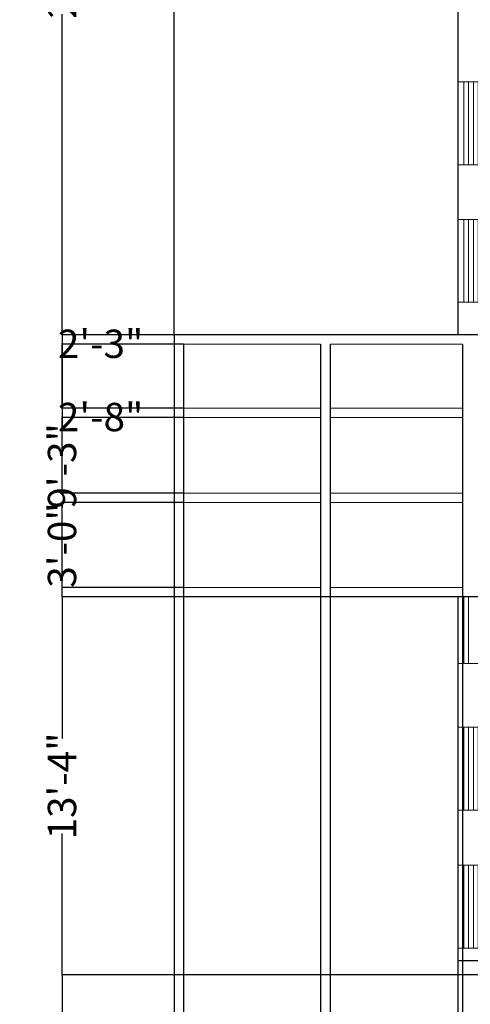
# Model space of a CAD drawing. Units: inches. Extents: x 1146 to 2917, y 889 to 2437.
# Tile 11 of 13: x 2395 to 2585, y 1586 to 2003. Entities that reach past the tile are written whole.
import ezdxf

# ---------------------------------------------------------------- set-up
doc = ezdxf.new("R2010")
doc.units = ezdxf.units.IN
doc.header["$MEASUREMENT"] = 0
for name, color, linetype, lineweight in [('A-ANNO-DIMS', 2, 'Continuous', 18), ('A-ELEV', 7, 'Continuous', 30), ('A-ELEV-GLAZ', 5, 'Continuous', 18), ('A-ELEV-ORNM', 8, 'Continuous', 18)]:
    doc.layers.add(name, color=color, linetype=linetype, lineweight=lineweight)
doc.styles.get("Standard").update_dxf_attribs({"font": 'arial.ttf'})
doc.dimstyles.get("Standard").update_dxf_attribs({"dimtxt": 12, "dimasz": 0.18, "dimexe": 0.18, "dimexo": 0.0625, "dimgap": 0.09, "dimtad": 0, "dimtoh": 1, "dimdec": 1, "dimzin": 0, "dimdsep": 46, "dimlunit": 4, "dimtxsty": 'Standard', "dimcen": 0.09, "dimadec": 0, "dimazin": 0, "dimtfac": 1, "dimtdec": 1, "dimtofl": 0, "dimtmove": 0, "dimatfit": 3, "dimfxl": 1, "dimtolj": 1, "dimtzin": 0, "dimarcsym": 0})

# ---------------------------------------------------------------- blocks, each defined once
blk = doc.blocks.new('PARAPET-LOUVER')
for p, q in [((2.58, 0), (2.58, 35.13)), ((4.58, 0), (4.58, 35.13)), ((6.58, 0), (6.58, 35.13)), ((8.58, 0), (8.58, 35.13))]:
    blk.add_line(p, q)
blk.add_lwpolyline([(0, 0), (11.07, 0), (11.07, 35.13), (0, 35.13)], close=True)
blk = doc.blocks.new('*D90')
at = {"layer": 'A-ANNO-DIMS', "color": 0, "lineweight": -2, "transparency": 16777216}
for p, q in [((2580.2, 1609.65), (2580.2, 1604.27)), ((2591.27, 1609.65), (2591.27, 1604.27)), ((2580.38, 1604.45), (2591.09, 1604.45)), ((2591.27, 1604.45), (2591.45, 1604.45))]:
    blk.add_line(p, q, dxfattribs=at)
at = {"layer": 'A-ANNO-DIMS', "color": 0, "transparency": 16777216}
for points in [[(2580.38, 1604.48), (2580.38, 1604.42), (2580.2, 1604.45)], [(2591.09, 1604.48), (2591.09, 1604.42), (2591.27, 1604.45)]]:
    blk.add_solid(points, dxfattribs=at)
at = {"layer": 'Defpoints', "color": 0, "transparency": 16777216}
for p in [(2580.2, 1609.72), (2591.27, 1609.72), (2591.27, 1604.45)]:
    blk.add_point(p, dxfattribs=at)
at = {"layer": 'A-ANNO-DIMS', "color": 0, "transparency": 16777216, "insert": (2632.77, 1604.45), "char_height": 12, "attachment_point": 5}
blk.add_mtext('\\A1;0\'-11" TYP.', dxfattribs=at)
blk = doc.blocks.new('*D122')
at = {"layer": 'A-ANNO-DIMS', "color": 0, "lineweight": -2, "transparency": 16777216}
for p, q in [((2460.2, 1869.45), (2460.2, 2418.97)), ((2460.38, 2418.79), (2585.4, 2418.79)), ((2752.02, 2418.79), (2627, 2418.79)), ((2752.2, 2371.45), (2752.2, 2418.97))]:
    blk.add_line(p, q, dxfattribs=at)
at = {"layer": 'A-ANNO-DIMS', "color": 0, "transparency": 16777216}
for points in [[(2460.38, 2418.82), (2460.38, 2418.76), (2460.2, 2418.79)], [(2752.02, 2418.82), (2752.02, 2418.76), (2752.2, 2418.79)]]:
    blk.add_solid(points, dxfattribs=at)
at = {"layer": 'Defpoints', "color": 0, "transparency": 16777216}
for p in [(2752.2, 2418.79), (2752.2, 2371.39), (2460.2, 1869.39)]:
    blk.add_point(p, dxfattribs=at)
at = {"layer": 'A-ANNO-DIMS', "color": 0, "transparency": 16777216, "insert": (2606.2, 2418.79), "char_height": 12, "attachment_point": 5}
blk.add_mtext('\\A1;24\'-4"', dxfattribs=at)
blk = doc.blocks.new('*D125')
at = {"layer": 'A-ANNO-DIMS', "color": 0, "lineweight": -2, "transparency": 16777216}
for p, q in [((2460.14, 1758.39), (2412.62, 1758.39)), ((2412.8, 1758.21), (2412.8, 1698.53)), ((2412.8, 1598.57), (2412.8, 1658.26)), ((2580.14, 1598.39), (2412.62, 1598.39))]:
    blk.add_line(p, q, dxfattribs=at)
at = {"layer": 'A-ANNO-DIMS', "color": 0, "transparency": 16777216}
for points in [[(2412.77, 1758.21), (2412.83, 1758.21), (2412.8, 1758.39)], [(2412.77, 1598.57), (2412.83, 1598.57), (2412.8, 1598.39)]]:
    blk.add_solid(points, dxfattribs=at)
at = {"layer": 'Defpoints', "color": 0, "transparency": 16777216}
for p in [(2412.8, 1758.39), (2460.2, 1758.39), (2580.2, 1598.39)]:
    blk.add_point(p, dxfattribs=at)
at = {"layer": 'A-ANNO-DIMS', "color": 0, "transparency": 16777216, "insert": (2412.8, 1678.39), "char_height": 12, "attachment_point": 5, "rotation": 90}
blk.add_mtext('\\A1;13\'-4"', dxfattribs=at)
blk = doc.blocks.new('*D126')
at = {"layer": 'A-ANNO-DIMS', "color": 0, "lineweight": -2, "transparency": 16777216}
for p, q in [((2460.14, 1869.39), (2412.62, 1869.39)), ((2412.8, 1869.21), (2412.8, 1829.93)), ((2412.8, 1758.57), (2412.8, 1797.85)), ((2460.14, 1758.39), (2412.62, 1758.39))]:
    blk.add_line(p, q, dxfattribs=at)
at = {"layer": 'A-ANNO-DIMS', "color": 0, "transparency": 16777216}
for points in [[(2412.77, 1869.21), (2412.83, 1869.21), (2412.8, 1869.39)], [(2412.77, 1758.57), (2412.83, 1758.57), (2412.8, 1758.39)]]:
    blk.add_solid(points, dxfattribs=at)
at = {"layer": 'Defpoints', "color": 0, "transparency": 16777216}
for p in [(2412.8, 1869.39), (2460.2, 1869.39), (2460.2, 1758.39)]:
    blk.add_point(p, dxfattribs=at)
at = {"layer": 'A-ANNO-DIMS', "color": 0, "transparency": 16777216, "insert": (2412.8, 1813.89), "char_height": 12, "attachment_point": 5, "rotation": 90}
blk.add_mtext('\\A1;9\'-3"', dxfattribs=at)
blk = doc.blocks.new('*D127')
at = {"layer": 'A-ANNO-DIMS', "color": 0, "lineweight": -2, "transparency": 16777216}
for p, q in [((2580.14, 2182.39), (2412.62, 2182.39)), ((2412.8, 2182.21), (2412.8, 2046.7)), ((2412.8, 1869.57), (2412.8, 2005.09)), ((2460.14, 1869.39), (2412.62, 1869.39))]:
    blk.add_line(p, q, dxfattribs=at)
at = {"layer": 'A-ANNO-DIMS', "color": 0, "transparency": 16777216}
for points in [[(2412.77, 2182.21), (2412.83, 2182.21), (2412.8, 2182.39)], [(2412.77, 1869.57), (2412.83, 1869.57), (2412.8, 1869.39)]]:
    blk.add_solid(points, dxfattribs=at)
at = {"layer": 'Defpoints', "color": 0, "transparency": 16777216}
for p in [(2412.8, 2182.39), (2580.2, 2182.39), (2460.2, 1869.39)]:
    blk.add_point(p, dxfattribs=at)
at = {"layer": 'A-ANNO-DIMS', "color": 0, "transparency": 16777216, "insert": (2412.8, 2025.89), "char_height": 12, "attachment_point": 5, "rotation": 90}
blk.add_mtext('\\A1;26\'-1"', dxfattribs=at)
blk = doc.blocks.new('*D128')
at = {"layer": 'A-ANNO-DIMS', "color": 0, "lineweight": -2, "transparency": 16777216}
for p, q in [((2580.2, 1598.33), (2580.2, 1384.31)), ((2752.2, 1431.83), (2752.2, 1384.31)), ((2580.38, 1384.49), (2646.06, 1384.49)), ((2752.02, 1384.49), (2686.34, 1384.49))]:
    blk.add_line(p, q, dxfattribs=at)
at = {"layer": 'A-ANNO-DIMS', "color": 0, "transparency": 16777216}
for points in [[(2580.38, 1384.52), (2580.38, 1384.46), (2580.2, 1384.49)], [(2752.02, 1384.52), (2752.02, 1384.46), (2752.2, 1384.49)]]:
    blk.add_solid(points, dxfattribs=at)
at = {"layer": 'Defpoints', "color": 0, "transparency": 16777216}
for p in [(2580.2, 1598.39), (2752.2, 1431.89), (2752.2, 1384.49)]:
    blk.add_point(p, dxfattribs=at)
at = {"layer": 'A-ANNO-DIMS', "color": 0, "transparency": 16777216, "insert": (2666.2, 1384.49), "char_height": 12, "attachment_point": 5}
blk.add_mtext('\\A1;14\'-4"', dxfattribs=at)
blk = doc.blocks.new('*D129')
at = {"layer": 'A-ANNO-DIMS', "color": 0, "lineweight": -2, "transparency": 16777216}
for p, q in [((2580.14, 1598.39), (2412.62, 1598.39)), ((2412.8, 1598.21), (2412.8, 1553.92)), ((2412.8, 1432.07), (2412.8, 1476.36)), ((2752.14, 1431.89), (2412.62, 1431.89))]:
    blk.add_line(p, q, dxfattribs=at)
at = {"layer": 'A-ANNO-DIMS', "color": 0, "transparency": 16777216}
for points in [[(2412.77, 1598.21), (2412.83, 1598.21), (2412.8, 1598.39)], [(2412.77, 1432.07), (2412.83, 1432.07), (2412.8, 1431.89)]]:
    blk.add_solid(points, dxfattribs=at)
at = {"layer": 'Defpoints', "color": 0, "transparency": 16777216}
for p in [(2580.2, 1598.39), (2412.8, 1431.89), (2752.2, 1431.89)]:
    blk.add_point(p, dxfattribs=at)
at = {"layer": 'A-ANNO-DIMS', "color": 0, "transparency": 16777216, "insert": (2412.8, 1515.14), "char_height": 12, "attachment_point": 5, "rotation": 90}
blk.add_mtext('\\A1;13\'-10 1/2"', dxfattribs=at)
blk = doc.blocks.new('*D130')
at = {"layer": 'A-ANNO-DIMS', "color": 0, "lineweight": -2, "transparency": 16777216}
for p, q in [((2464.14, 1798.39), (2412.62, 1798.39)), ((2412.8, 1798.21), (2412.8, 1796.43)), ((2412.8, 1762.57), (2412.8, 1764.36)), ((2464.14, 1762.39), (2412.62, 1762.39))]:
    blk.add_line(p, q, dxfattribs=at)
at = {"layer": 'A-ANNO-DIMS', "color": 0, "transparency": 16777216}
for points in [[(2412.77, 1798.21), (2412.83, 1798.21), (2412.8, 1798.39)], [(2412.77, 1762.57), (2412.83, 1762.57), (2412.8, 1762.39)]]:
    blk.add_solid(points, dxfattribs=at)
at = {"layer": 'Defpoints', "color": 0, "transparency": 16777216}
for p in [(2412.8, 1798.39), (2464.2, 1798.39), (2464.2, 1762.39)]:
    blk.add_point(p, dxfattribs=at)
at = {"layer": 'A-ANNO-DIMS', "color": 0, "transparency": 16777216, "insert": (2412.8, 1780.39), "char_height": 12, "attachment_point": 5, "rotation": 90}
blk.add_mtext('\\A1;3\'-0"', dxfattribs=at)
blk = doc.blocks.new('*D131')
at = {"layer": 'A-ANNO-DIMS', "color": 0, "lineweight": -2, "transparency": 16777216}
for p, q in [((2464.14, 1834.39), (2412.62, 1834.39)), ((2412.8, 1834.39), (2412.8, 1834.57)), ((2412.8, 1834.57), (2412.98, 1834.57)), ((2412.8, 1802.57), (2412.8, 1834.21)), ((2464.14, 1802.39), (2412.62, 1802.39))]:
    blk.add_line(p, q, dxfattribs=at)
at = {"layer": 'A-ANNO-DIMS', "color": 0, "transparency": 16777216}
for points in [[(2412.77, 1834.21), (2412.83, 1834.21), (2412.8, 1834.39)], [(2412.77, 1802.57), (2412.83, 1802.57), (2412.8, 1802.39)]]:
    blk.add_solid(points, dxfattribs=at)
at = {"layer": 'Defpoints', "color": 0, "transparency": 16777216}
for p in [(2412.8, 1834.39), (2464.2, 1834.39), (2464.2, 1802.39)]:
    blk.add_point(p, dxfattribs=at)
at = {"layer": 'A-ANNO-DIMS', "color": 0, "transparency": 16777216, "insert": (2429.12, 1834.57), "char_height": 12, "attachment_point": 5}
blk.add_mtext('\\A1;2\'-8"', dxfattribs=at)
blk = doc.blocks.new('*D132')
at = {"layer": 'A-ANNO-DIMS', "color": 0, "lineweight": -2, "transparency": 16777216}
for p, q in [((2464.14, 1865.39), (2412.62, 1865.39)), ((2412.8, 1865.39), (2412.8, 1865.57)), ((2412.8, 1865.57), (2412.98, 1865.57)), ((2412.8, 1838.57), (2412.8, 1865.21)), ((2464.14, 1838.39), (2412.62, 1838.39))]:
    blk.add_line(p, q, dxfattribs=at)
at = {"layer": 'A-ANNO-DIMS', "color": 0, "transparency": 16777216}
for points in [[(2412.77, 1865.21), (2412.83, 1865.21), (2412.8, 1865.39)], [(2412.77, 1838.57), (2412.83, 1838.57), (2412.8, 1838.39)]]:
    blk.add_solid(points, dxfattribs=at)
at = {"layer": 'Defpoints', "color": 0, "transparency": 16777216}
for p in [(2412.8, 1865.39), (2464.2, 1865.39), (2464.2, 1838.39)]:
    blk.add_point(p, dxfattribs=at)
at = {"layer": 'A-ANNO-DIMS', "color": 0, "transparency": 16777216, "insert": (2429.12, 1865.57), "char_height": 12, "attachment_point": 5}
blk.add_mtext('\\A1;2\'-3"', dxfattribs=at)
blk = doc.blocks.new('*D133')
at = {"layer": 'A-ANNO-DIMS', "color": 0, "lineweight": -2, "transparency": 16777216}
for p, q in [((2464.2, 1865.33), (2464.2, 1384.31)), ((2522.2, 1865.33), (2522.2, 1384.31)), ((2464.38, 1384.49), (2472.26, 1384.49)), ((2522.02, 1384.49), (2514.14, 1384.49))]:
    blk.add_line(p, q, dxfattribs=at)
at = {"layer": 'A-ANNO-DIMS', "color": 0, "transparency": 16777216}
for points in [[(2464.38, 1384.52), (2464.38, 1384.46), (2464.2, 1384.49)], [(2522.02, 1384.52), (2522.02, 1384.46), (2522.2, 1384.49)]]:
    blk.add_solid(points, dxfattribs=at)
at = {"layer": 'Defpoints', "color": 0, "transparency": 16777216}
for p in [(2464.2, 1865.39), (2522.2, 1865.39), (2522.2, 1384.49)]:
    blk.add_point(p, dxfattribs=at)
at = {"layer": 'A-ANNO-DIMS', "color": 0, "transparency": 16777216, "insert": (2493.2, 1384.49), "char_height": 12, "attachment_point": 5}
blk.add_mtext('\\A1;4\'-10"', dxfattribs=at)
blk = doc.blocks.new('*D134')
at = {"layer": 'A-ANNO-DIMS', "color": 0, "lineweight": -2, "transparency": 16777216}
for p, q in [((2526.2, 1865.33), (2526.2, 1384.31)), ((2582.2, 1865.33), (2582.2, 1384.31)), ((2526.38, 1384.49), (2537.92, 1384.49)), ((2582.02, 1384.49), (2570.48, 1384.49))]:
    blk.add_line(p, q, dxfattribs=at)
at = {"layer": 'A-ANNO-DIMS', "color": 0, "transparency": 16777216}
for points in [[(2526.38, 1384.52), (2526.38, 1384.46), (2526.2, 1384.49)], [(2582.02, 1384.52), (2582.02, 1384.46), (2582.2, 1384.49)]]:
    blk.add_solid(points, dxfattribs=at)
at = {"layer": 'Defpoints', "color": 0, "transparency": 16777216}
for p in [(2526.2, 1865.39), (2582.2, 1865.39), (2582.2, 1384.49)]:
    blk.add_point(p, dxfattribs=at)
at = {"layer": 'A-ANNO-DIMS', "color": 0, "transparency": 16777216, "insert": (2554.2, 1384.49), "char_height": 12, "attachment_point": 5}
blk.add_mtext('\\A1;4\'-8"', dxfattribs=at)
blk = doc.blocks.new('*D135')
at = {"layer": 'A-ANNO-DIMS', "color": 0, "lineweight": -2, "transparency": 16777216}
for p, q in [((2460.2, 1869.33), (2460.2, 1384.31)), ((2464.2, 1865.33), (2464.2, 1384.31)), ((2460.38, 1384.49), (2464.02, 1384.49)), ((2464.2, 1384.49), (2464.38, 1384.49))]:
    blk.add_line(p, q, dxfattribs=at)
at = {"layer": 'A-ANNO-DIMS', "color": 0, "transparency": 16777216}
for points in [[(2460.38, 1384.52), (2460.38, 1384.46), (2460.2, 1384.49)], [(2464.02, 1384.52), (2464.02, 1384.46), (2464.2, 1384.49)]]:
    blk.add_solid(points, dxfattribs=at)
at = {"layer": 'Defpoints', "color": 0, "transparency": 16777216}
for p in [(2460.2, 1869.39), (2464.2, 1865.39), (2464.2, 1384.49)]:
    blk.add_point(p, dxfattribs=at)
at = {"layer": 'A-ANNO-DIMS', "color": 0, "transparency": 16777216, "insert": (2480.42, 1384.49), "char_height": 12, "attachment_point": 5}
blk.add_mtext('\\A1;0\'-4"', dxfattribs=at)

msp = doc.modelspace()

# ---------------------------------------------------------------- linework, layer by layer
at = {"layer": 'A-ELEV'}
for p, q in [((2580.2, 2182.39), (2580.2, 1869.39)), ((2688.2, 1869.39), (2460.2, 1869.39)), ((2460.2, 1869.39), (2460.2, 1758.39)), ((2688.2, 1758.39), (2460.2, 1758.39)), ((2580.2, 1758.39), (2580.2, 1598.39)), ((2688.2, 1598.39), (2580.2, 1598.39))]:
    msp.add_line(p, q, dxfattribs=at)
at = {"layer": 'A-ELEV-GLAZ'}
for p, q in [((2464.2, 1865.39), (2464.2, 1838.39)), ((2522.2, 1865.39), (2464.2, 1865.39)), ((2522.2, 1865.39), (2522.2, 1838.39)), ((2526.2, 1865.39), (2526.2, 1838.39)), ((2582.2, 1865.39), (2526.2, 1865.39)), ((2582.2, 1865.39), (2582.2, 1838.39)), ((2522.2, 1838.39), (2464.2, 1838.39)), ((2582.2, 1838.39), (2526.2, 1838.39)), ((2522.2, 1834.39), (2464.2, 1834.39)), ((2464.2, 1834.39), (2464.2, 1802.39)), ((2522.2, 1834.39), (2522.2, 1802.39)), ((2582.2, 1834.39), (2526.2, 1834.39)), ((2526.2, 1834.39), (2526.2, 1802.39)), ((2582.2, 1834.39), (2582.2, 1802.39)), ((2522.2, 1802.39), (2464.2, 1802.39)), ((2582.2, 1802.39), (2526.2, 1802.39)), ((2522.2, 1798.39), (2464.2, 1798.39)), ((2464.2, 1798.39), (2464.2, 1762.39)), ((2522.2, 1798.39), (2522.2, 1762.39)), ((2582.2, 1798.39), (2526.2, 1798.39)), ((2526.2, 1798.39), (2526.2, 1762.39)), ((2582.2, 1798.39), (2582.2, 1762.39)), ((2522.2, 1762.39), (2464.2, 1762.39)), ((2582.2, 1762.39), (2526.2, 1762.39))]:
    msp.add_line(p, q, dxfattribs=at)
at = {"layer": 'A-ELEV-ORNM'}
for p, q in [((2582.78, 1730.24), (2582.78, 1758.39)), ((2584.78, 1730.24), (2584.78, 1758.39))]:
    msp.add_line(p, q, dxfattribs=at)
msp.add_lwpolyline([(2580.2, 1758.39), (2580.2, 1730.24), (2591.27, 1730.24), (2591.27, 1758.39)], dxfattribs=at)

# ---------------------------------------------------------------- block references
for p in [(2580.2, 1941.29), (2580.2, 1883.13), (2580.2, 1668.12), (2580.2, 1609.72)]:
    msp.add_blockref('PARAPET-LOUVER', p, dxfattribs=at)

# ---------------------------------------------------------------- dimensions: what is measured, and where the dimension line sits
at = {"layer": 'A-ANNO-DIMS'}
for base, p1, p2, picture, middle in [((2752.2, 2418.79), (2460.2, 1869.39), (2752.2, 2371.39), '*D122', (2606.2, 2418.79)), ((2464.2, 1384.49), (2460.2, 1869.39), (2464.2, 1865.39), '*D135', (2480.42, 1384.49)), ((2522.2, 1384.49), (2464.2, 1865.39), (2522.2, 1865.39), '*D133', (2493.2, 1384.49)), ((2582.2, 1384.49), (2526.2, 1865.39), (2582.2, 1865.39), '*D134', (2554.2, 1384.49)), ((2752.2, 1384.49), (2580.2, 1598.39), (2752.2, 1431.89), '*D128', (2666.2, 1384.49))]:
    dim = msp.add_linear_dim(base=base, p1=p1, p2=p2, dimstyle='Standard', override={"dimdec": 1, "dimlfac": 1, "dimrnd": 0, "dimzin": 1, "dimdsep": 46, "dimlunit": 4, "dimfrac": 2}, dxfattribs=at)
    dim.commit()
    dim.dimension.update_dxf_attribs({"geometry": picture, "text_midpoint": middle})
for base, p1, p2, picture, middle in [((2412.8, 2182.39), (2460.2, 1869.39), (2580.2, 2182.39), '*D127', (2412.8, 2025.89)), ((2412.8, 1865.39), (2464.2, 1838.39), (2464.2, 1865.39), '*D132', (2429.12, 1865.57)), ((2412.8, 1869.39), (2460.2, 1758.39), (2460.2, 1869.39), '*D126', (2412.8, 1813.89)), ((2412.8, 1834.39), (2464.2, 1802.39), (2464.2, 1834.39), '*D131', (2429.12, 1834.57)), ((2412.8, 1798.39), (2464.2, 1762.39), (2464.2, 1798.39), '*D130', (2412.8, 1780.39)), ((2412.8, 1758.39), (2580.2, 1598.39), (2460.2, 1758.39), '*D125', (2412.8, 1678.39)), ((2412.8, 1431.89), (2580.2, 1598.39), (2752.2, 1431.89), '*D129', (2412.8, 1515.14))]:
    dim = msp.add_linear_dim(base=base, p1=p1, p2=p2, angle=90, dimstyle='Standard', override={"dimdec": 1, "dimlfac": 1, "dimrnd": 0, "dimzin": 1, "dimdsep": 46, "dimlunit": 4, "dimfrac": 2}, dxfattribs=at)
    dim.commit()
    dim.dimension.update_dxf_attribs({"geometry": picture, "text_midpoint": middle})
dim = msp.add_linear_dim(base=(2591.27, 1604.45), p1=(2580.2, 1609.72), p2=(2591.27, 1609.72), text='<> TYP.', dimstyle='Standard', override={"dimdec": 1, "dimlfac": 1, "dimrnd": 0, "dimzin": 1, "dimdsep": 46, "dimlunit": 4, "dimfrac": 2}, dxfattribs=at)
dim.commit()
dim.dimension.update_dxf_attribs({"geometry": '*D90', "text_midpoint": (2632.77, 1604.45)})

doc.saveas('drawing.dxf')
